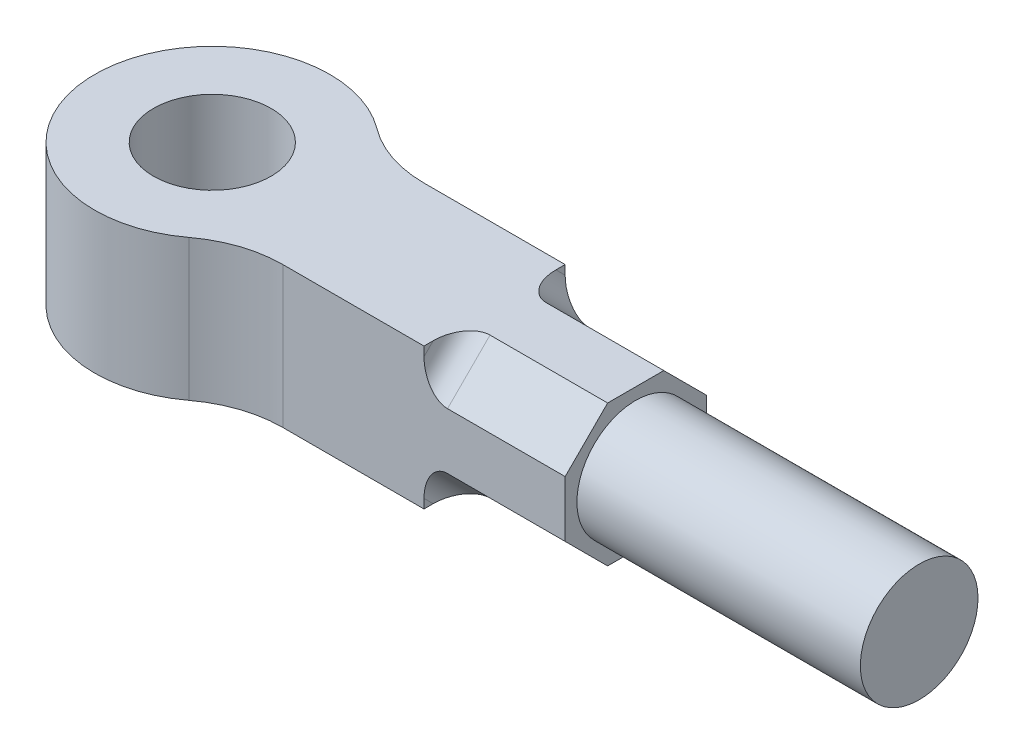
from build123d import *

# Parameters (mm, degrees)
EYE_PROFILE_SKETCH_R   = 25
EYE_BLOCK_60MM_DEPTH   = 60
NECK_FLATS_CUT_DEPTH   = 60
SKETCH2_4_R            = 25
ROD_BOSS_120_5MM_DEPTH = 120.5
NECK_FILLET_R10_R      = 10


with BuildPart() as part:
    # Eye Profile Sketch → Eye Block 60mm (new body)
    with BuildSketch(Plane(origin=(0, 0, 0), x_dir=(1, 0, 0), z_dir=(0, 1, 0))):
        with BuildLine():
            Line((60, 30), (180, 30))
            Line((180, 30), (180, -30))
            Line((180, -30), (60, -30))
            ThreePointArc((60, -30), (44.188611699, -32.565835097), (30, -40))
            ThreePointArc((30, -40), (-50, 0), (30, 40))
            ThreePointArc((30, 40), (44.188611699, 32.565835097), (60, 30))
        make_face()
        with Locations(Location((0, 0, 0), (0, 0, 270))):
            Circle(EYE_PROFILE_SKETCH_R, mode=Mode.SUBTRACT)
    extrude(amount=EYE_BLOCK_60MM_DEPTH)

    # Neck and Rod Sketch → Neck Flats Cut (cut)
    with BuildSketch(Plane(origin=(180, 0, 0), x_dir=(0, 0, -1), z_dir=(1, 0, 0))):
        Polygon((-11.94, 60), (-30, 60), (-30, 41.94), align=None)
        Polygon((30, 60), (11.94, 60), (30, 41.94), align=None)
        Polygon((-11.94, 0), (-30, 18.06), (-30, 0), align=None)
        Polygon((30, 0), (30, 18.06), (11.94, 0), align=None)
    extrude(amount=-NECK_FLATS_CUT_DEPTH, mode=Mode.SUBTRACT)

    # Sketch2_4 → Rod Boss 120.5mm (add)
    with BuildSketch(Plane(origin=(180, 0, 0), x_dir=(0, 0, -1), z_dir=(1, 0, 0))):
        with Locations((0, 30)):
            Circle(SKETCH2_4_R)
    extrude(amount=ROD_BOSS_120_5MM_DEPTH)

    # Neck Fillet R10
    neck_fillet_r10_edges = [part.edges().sort_by_distance(p)[0] for p in [
        (120, 50.97, -20.97),
        (120, 9.03, 20.97),
        (120, 9.03, -20.97),
        (120, 50.97, 20.97),
    ]]
    fillet(neck_fillet_r10_edges, radius=NECK_FILLET_R10_R)


solid = part.part
